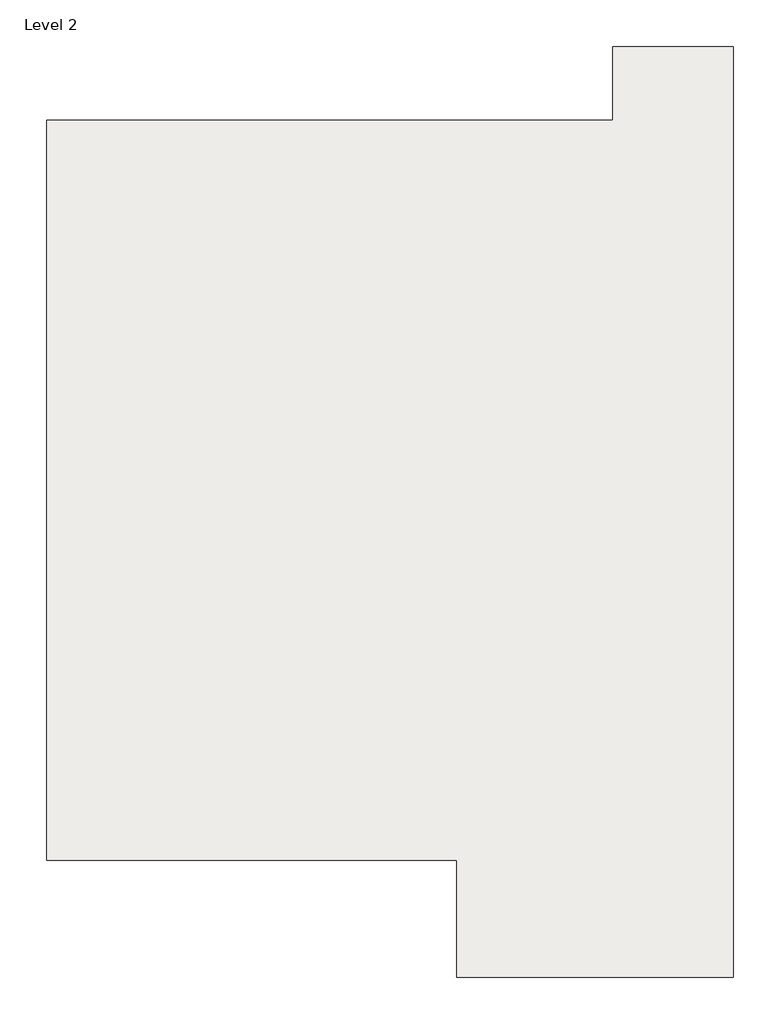
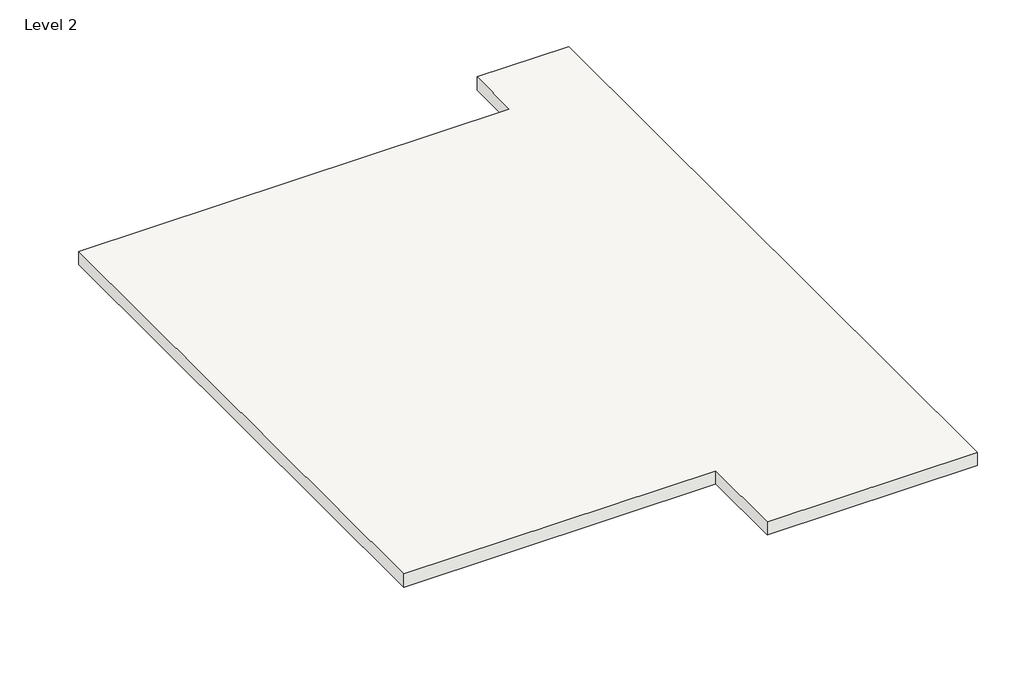
# One storey: 1 roof.
"""IFC4 building model written with IfcOpenShell, lengths in millimetres."""

from ifc_helpers import new_model, si_unit, frame, origin, place, context, project, spatial, polyline, outline, extrude, element, save

model = new_model("IFC4")

# Units and contexts
model_context = context("Model", 3, world=origin())
ifc_project = project(units=[si_unit("LENGTHUNIT", "METRE", prefix="MILLI")], contexts=[model_context])

# Site, building, storey
site = spatial("IfcSite", under=ifc_project)
building = spatial("IfcBuilding", under=site)
storey = spatial("IfcBuildingStorey", under=building, Name="Level 2", Elevation=3048.0)

# Roof
placement = place(None, origin())
element("IfcRoof", 1, ObjectType="Generic - 12\"", at=placement, inside=storey, context=model_context, shape_type="SweptSolid", body=[
    extrude(outline(polyline([(-8546.1557202, 14258.0245992), (813.7442798, 14258.0245992), (813.7442798, 15477.2245992), (2807.6442798, 15477.2245992), (2807.6442798, 84.8245992), (-1764.3557202, 84.8245992), (-1764.3557202, 2021.5745992), (-8546.1557202, 2021.5745992), (-8546.1557202, 14258.0245992)])), frame((0.0, 0.0, 3048.0), z_axis=(0.0, 0.0, 1.0), x_axis=(1.0, 0.0, 0.0)), (0.0, 0.0, 1.0), 304.8),
])

save(model, "model.ifc")

# Revit data of these elements
# Type "Generic - 12\""
#   Assembly Code = "B1020"
#   Layers, outside or top first: 1' - 0" "Brick, Soldier Course" (function 1)
# Element 1 (IfcRoof, "Generic - 12\"")
#   built-in parameter 1001705 = 11 (stored number, unit not read)
#   built-in parameter 1001710 = 33615
#   Phase Created = New Construction
#   Materials on its faces: "Brick, Soldier Course"
# Materials
#   "Brick, Soldier Course": class "Masonry", colour RGB 170 98 104, transparency 0, Description = "Common brick soldier coursed", Cost = 0
